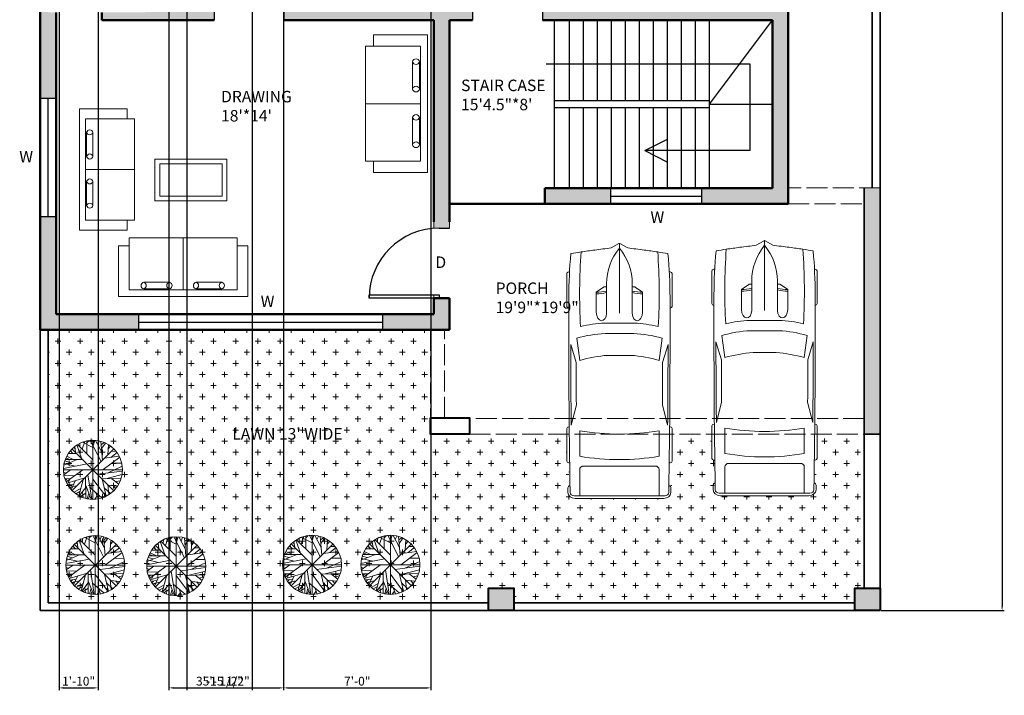
# Model space of a CAD drawing. Units: inches. Extents: x 2101 to 2663, y 1144 to 2069.
# Tile 1 of 4: x 2101 to 2663, y 1144 to 1530. Entities that reach past the tile are written whole.
import ezdxf

# ---------------------------------------------------------------- set-up
doc = ezdxf.new("R2010")
doc.units = ezdxf.units.IN
doc.linetypes.add('ACAD_ISO02W100', pattern=[15, 12, -3])
for name, color, linetype, lineweight in [('A-ANNO-DIMS', 2, 'Continuous', 18), ('A-ANNO-TEXT', 7, 'Continuous', 18), ('A-AREA-IDEN', 7, 'Continuous', 25), ('A-COLS', 7, 'Continuous', 40), ('A-FLOR-STRS', 7, 'Continuous', 25), ('A-WALL-OVHD', 240, 'ACAD_ISO02W100', 18), ('A-WALL-PATT', 240, 'Continuous', 13), ('C-PKNG-VEHI', 142, 'Continuous', 18), ('C-PROP', 7, 'Continuous', 35), ('door', 52, 'Continuous', 25), ('fur', 142, 'Continuous', 18), ('L-PLNT-PATT', 92, 'Continuous', 13), ('tree', 90, 'Continuous', 18), ('wall', 240, 'Continuous', 50), ('win', 150, 'Continuous', 25)]:
    doc.layers.add(name, color=color, linetype=linetype, lineweight=lineweight)
doc.styles.get("Standard").update_dxf_attribs({"font": 'arial.ttf'})
doc.dimstyles.new('ISO-25', dxfattribs={"dimtxt": 5, "dimasz": 2.5, "dimexe": 1.25, "dimexo": 0.625, "dimtad": 1, "dimdec": 0, "dimlunit": 4, "dimtxsty": 'Standard', "dimcen": 2.5, "dimadec": 0, "dimazin": 0, "dimtfac": 1, "dimtdec": 0, "dimtmove": 0, "dimatfit": 3, "dimfxl": 1, "dimarcsym": 0})

# ---------------------------------------------------------------- blocks, each defined once
blk = doc.blocks.new('*U6')
for p, q in [((0, 59.9996), (0, -60)), ((-43.8768, 36.4326), (-44.405, 40.2696)), ((42, 42), (-42, -42)), ((42, -42), (-42, 42)), ((-40.1797, 44.558), (-36.4825, 43.2038)), ((-37.0107, 47.0408), (-35.25, 35.5298)), ((-32.6092, 50.4264), (-23.2782, 23.5674)), ((-31.2008, 51.1035), (-0.2149, 20.1818)), ((-26.4472, 46.5894), (-26.2712, 53.8116)), ((-22.0458, 42.0753), (-16.5881, 57.6486)), ((-21.1656, 55.8436), (-0.0388, 45.0094)), ((-12.5388, 54.9406), (-7.9613, 59.4546)), ((-12.3627, 32.1443), (-12.5388, 58.7776)), ((-5.3205, 59.6806), (16.5105, 16.7963)), ((2.426, 54.9406), (-1.4472, 59.9056)), ((0.4894, 48.6208), (3.6584, 59.6806)), ((18.2711, 35.5298), (5.419, 59.6806)), ((9.8203, 51.5549), (12.8133, 58.5516)), ((19.6795, 19.5047), (16.3344, 57.6486)), ((17.0387, 51.1035), (23.2006, 55.1666)), ((17.7429, 43.6552), (25.4894, 54.2636)), ((31.6513, 50.8778), (30.2429, 30.5643)), ((31.1232, 42.5267), (35.8767, 48.1693)), ((-32.2571, 20.6333), (-59.1937, 9.348)), ((-56.0247, 20.859), (-20.8134, 20.859)), ((-54.7923, 24.4702), (-47.75, 21.0847)), ((-53.2078, 27.4044), (-40.1797, 20.859)), ((-49.8627, 32.8214), (-32.7853, 32.8214)), ((-45.8134, 38.2383), (-40.5318, 33.0471)), ((54.3626, 25.3731), (20.9119, 0.3198)), ((23.3767, 23.3417), (53.3063, 27.4044)), ((36.2288, 25.1474), (48.9049, 35.0784)), ((37.1091, 37.1098), (46.6161, 37.5612)), ((-59.7219, 2.8025), (-12.0106, 12.0565)), ((-58.6656, 12.7336), (-35.9543, 7.5424)), ((-57.081, 17.9248), (-47.0458, 14.7649)), ((-54.6162, -24.7335), (-20.2853, 0.0941)), ((29.3626, -6.6771), (59.4682, 7.091)), ((38.5175, 13.4107), (58.2359, 13.6364)), ((-60, 0), (60, 0)), ((-59.7219, -4.8714), (-54.2641, -6.6771)), ((-45.2853, -0.1316), (-59.0177, -10.0627)), ((-58.4895, -12.3197), (-36.4825, -11.6426)), ((-57.081, -18.4138), (-45.2853, -17.9624)), ((-52.6797, -18.188), (-55.4966, -22.0251)), ((-53.2078, -27.442), (-16.7641, -16.6081)), ((-47.2219, -19.3166), (-50.2148, -26.3135)), ((-14.8275, -15.0282), (-14.6515, -57.6865)), ((-10.074, -10.0627), (-2.5036, -59.7178)), ((-0.0388, -19.0909), (25.8415, -53.8495)), ((9.2922, -9.1598), (59.6443, -2.8401)), ((18.6232, -18.6394), (26.7218, -53.3981)), ((18.7992, -18.6394), (57.3556, -17.2853)), ((26.3697, -18.4138), (58.9401, -9.8369)), ((38.1654, -18.188), (52.426, -29.0219)), ((-38.9472, -29.0219), (-51.4472, -30.6018)), ((-46.5177, -30.1504), (-49.5106, -33.536)), ((-32.4331, -32.4075), (-48.1021, -35.5674)), ((-43.7008, -34.6645), (-46.6937, -37.373)), ((-35.9543, -22.4765), (-44.0529, -40.5329)), ((-24.6867, -37.8244), (-38.7712, -45.7241)), ((-19.9331, -20.2194), (-28.5599, -52.721)), ((-14.6515, -36.2445), (-27.6797, -52.9467)), ((-14.6515, -32.1818), (-3.912, -59.4922)), ((-6.2008, -36.2445), (17.919, -57.0094)), ((22.8485, -36.4702), (35.3485, -48.4326)), ((30.419, -30.1504), (32.3556, -50.0125)), ((31.4753, -31.279), (49.6091, -33.3103)), ((41.5105, -32.6332), (46.088, -38.0501)), ((45.9119, -24.0564), (55.595, -22.2508)), ((-26.2712, -43.9185), (-34.7219, -48.6583)), ((-14.6515, -47.3041), (-25.0388, -54.3009)), ((-21.5177, -45.4984), (-19.9331, -56.1065)), ((-8.4895, -47.5298), (-11.4825, -58.5893)), ((-6.3768, -52.721), (-9.3698, -58.815)), ((8.4119, -53.1724), (3.8344, -59.4922)), ((5.9471, -46.6269), (10.5246, -58.5893)), ((24.7852, -44.8213), (23.0246, -54.978))]:
    blk.add_line(p, q)
blk.add_circle((0, 0), 60)
blk = doc.blocks.new('*U2')
for p, q in [((0, 0), (0, -6)), ((40, 0), (40, -6))]:
    blk.add_line(p, q)
blk.add_lwpolyline([(0, 0), (0, 40), (1.75, 40), (1.75, 0)], close=True)
blk.add_arc((0, 0), 40, 0, 90)
blk = doc.blocks.new('*U8')
for p, q in [((21.1, 37.41), (21.1, 36.83)), ((46.55, 38.89), (22.35, 38.89)), ((47.8, 37.39), (47.8, 37.41)), ((135.45, 37.07), (135.45, 37.41)), ((136.7, 38.89), (160.9, 38.89)), ((162.15, 37.41), (162.15, 36.77)), ((70.03, 31.54), (86.41, 29.35)), ((87.99, 31.87), (74.76, 35.92)), ((134.31, 35.6), (119.29, 31.78)), ((138.42, 29.35), (157.25, 29.35)), ((186.47, 29.35), (167.01, 29.35)), ((186.47, -33.5), (186.47, 33.5)), ((188.4, -32.76), (188.4, 32.76)), ((164.52, 26.39), (164.52, -26.39)), ((32.27, 11.63), (36.13, 17.17)), ((36.13, 17.17), (50.94, 17.17)), ((29.77, 9.51), (51.68, 9.51)), ((32.12, 9.51), (32.12, 11.15)), ((58.92, -10.77), (58.92, 10.77)), ((66.55, -10.53), (66.55, 10.53)), ((82.74, 8.5), (82.74, -8.5)), ((186.47, -10.53), (186.47, 10.53)), ((3.27, 6.13), (0.1, 0.41)), ((0, 0), (51.68, 0)), ((0.1, -0.41), (3.27, -6.13)), ((29.77, -9.51), (51.68, -9.51)), ((32.12, -9.51), (32.12, -11.15)), ((32.27, -11.63), (36.13, -17.17)), ((36.13, -17.17), (50.94, -17.17)), ((86.41, -29.35), (70.03, -31.54)), ((87.99, -31.87), (74.76, -35.92)), ((134.31, -35.6), (119.29, -31.78)), ((157.25, -29.35), (138.42, -29.35)), ((167.01, -29.35), (186.47, -29.35)), ((21.1, -37.41), (21.1, -36.83)), ((46.55, -38.89), (22.35, -38.89)), ((47.8, -37.39), (47.8, -37.41)), ((135.45, -37.07), (135.45, -37.41)), ((136.7, -38.89), (160.9, -38.89)), ((162.15, -37.41), (162.15, -36.77))]:
    blk.add_line(p, q)
for centre, major_axis, ratio, start_param, end_param in [((41.19, -490.86), (0, 528.23), 0.842304, 0.00281, 0.075598), ((22.35, 37.41), (0, -1.48), 0.842304, 3.141593, 4.712389), ((64.48, -10555.62), (0, 10593.03), 0.842304, -0.013397, 0.002797), ((46.55, 37.41), (0, 1.48), 0.842304, -1.570796, 0), ((136.7, 37.41), (0, -1.48), 0.842304, 3.141593, 4.712389), ((160.9, 37.41), (0, 1.48), 0.842304, -1.570796, 0), ((180.63, 35.84), (0, 2.22), 0.842304, -0.013017, 1.249894), ((64.48, -10556.36), (0, 10595.31), 0.842304, -0.013397, -0.013017), ((183.98, 33.5), (0, -2.96), 0.842304, 1.570796, 3.128196), ((183.98, 32.76), (0, -5.25), 0.842304, 1.570796, 3.128196), ((266.03, -27.52), (0, 313.31), 0.842304, 1.367076, 1.39176), ((37.47, -593.96), (0, -623.33), 0.842304, 3.096046, 3.200911), ((135.29, 5.39), (0, 81.77), 0.842304, 1.245306, 1.50788), ((64.48, -10555.62), (0, -10591.55), 0.842304, 3.133765, 3.140441), ((149.6, 2.8), (0, -79.58), 0.842304, 4.372215, 4.640744), ((95.79, -3666.35), (0, -3698.24), 0.842304, 3.134049, 3.144098), ((17.08, 0), (0, 147.02), 0.842304, 4.511394, 4.913384), ((35.91, 0), (0, 147.02), 0.842304, 4.511394, 4.913384), ((167.01, 26.39), (0, 2.96), 0.842304, 0, 1.570796), ((259.18, -27.52), (0, -305.3), 0.842304, 4.528606, 4.561838), ((134.4, 5.39), (0, -89.78), 0.842304, 4.449482, 4.652344), ((-204.49, 52.4), (0, -250.96), 0.842304, 1.385369, 1.434372), ((13.04, 17.01), (0, 27.42), 0.842304, 4.435146, 4.718221), ((14.2, 17.01), (0, 27.42), 0.842304, 4.435146, 4.718221), ((50.79, 13.34), (6.34, -0.36), 0.603834, -1.395552, 1.581315), ((29.77, -46.66), (0, 56.17), 0.842304, 0, 0.590319), ((32.75, 11.15), (0, 0.74), 0.842304, 0.879714, 1.570796), ((0.62, 0), (0, -0.74), 0.842304, 4.131459, 5.293319), ((-204.49, -52.4), (0, 250.96), 0.842304, -1.434372, -1.385369), ((29.77, 46.66), (0, 56.17), 0.842304, 2.551274, 3.141593), ((32.75, -11.15), (0, -0.74), 0.842304, 4.712389, 5.403472), ((13.04, -17.01), (0, -27.42), 0.842304, 1.564964, 1.848039), ((14.2, -17.01), (0, -27.42), 0.842304, 1.564964, 1.848039), ((134.4, -5.39), (0, -89.78), 0.842304, -1.510751, -1.307889), ((135.29, -5.39), (0, -81.77), 0.842304, -1.50788, -1.245306), ((149.6, -2.8), (0, -79.58), 0.842304, -1.499151, -1.230623), ((259.18, 27.52), (0, 305.3), 0.842304, 1.721348, 1.754579), ((266.03, 27.52), (0, 313.31), 0.842304, 1.749832, 1.774517), ((37.47, 593.96), (0, -623.33), 0.842304, -0.059319, 0.045547), ((167.01, -26.39), (0, -2.96), 0.842304, 4.712389, 6.283185), ((41.19, 490.86), (0, -528.23), 0.842304, -0.075598, -0.00281), ((64.48, 10555.62), (0, -10591.55), 0.842304, 0.001152, 0.007828), ((95.79, 3666.35), (0, -3698.24), 0.842304, -0.002505, 0.007544), ((183.98, -33.5), (0, 2.96), 0.842304, 3.15499, 4.712389), ((183.98, -32.76), (0, -5.25), 0.842304, 0.013397, 1.570796), ((22.35, -37.41), (0, 1.48), 0.842304, 1.570796, 3.141593), ((64.48, 10555.62), (0, 10593.03), 0.842304, 3.138796, 3.15499), ((46.55, -37.41), (0, -1.48), 0.842304, 0, 1.570796), ((136.7, -37.41), (0, -1.48), 0.842304, -1.570796, 0), ((160.9, -37.41), (0, 1.48), 0.842304, 3.141593, 4.712389), ((180.63, -35.84), (0, -2.22), 0.842304, -1.249894, 0.013017), ((64.48, 10556.36), (0, 10595.31), 0.842304, 3.15461, 3.15499)]:
    blk.add_ellipse(centre, major_axis=major_axis, ratio=ratio, start_param=start_param, end_param=end_param)
at = {"extrusion": (0, 0, -1)}
blk.add_ellipse((50.79, -13.34), major_axis=(6.34, 0.36), ratio=0.603834, start_param=-1.395552, end_param=1.581315, dxfattribs=at)
blk = doc.blocks.new('*D10')
at = {"layer": 'A-ANNO-DIMS', "color": 0, "lineweight": -2, "transparency": 16777216}
for p, q in [((2593.02, 2003.65), (2663.42, 2003.65)), ((2662.17, 2001.15), (2662.17, 1194.65)), ((2593.02, 1192.15), (2663.42, 1192.15))]:
    blk.add_line(p, q, dxfattribs=at)
at = {"layer": 'A-ANNO-DIMS', "color": 0, "lineweight": 100, "transparency": 16777216}
for points in [[(2661.75, 2001.15), (2662.59, 2001.15), (2662.17, 2003.65)], [(2661.75, 1194.65), (2662.59, 1194.65), (2662.17, 1192.15)]]:
    blk.add_solid(points, dxfattribs=at)
at = {"layer": 'Defpoints', "color": 0, "lineweight": 100, "transparency": 16777216}
for p in [(2592.39, 2003.65), (2592.39, 1192.15), (2662.17, 1192.15)]:
    blk.add_point(p, dxfattribs=at)
at = {"layer": 'A-ANNO-DIMS', "color": 0, "transparency": 16777216, "insert": (2658.99, 1597.9), "char_height": 5, "attachment_point": 5, "rotation": 90}
blk.add_mtext('67\'-8"', dxfattribs=at)
blk = doc.blocks.new('*D31')
at = {"layer": 'A-ANNO-DIMS', "color": 0, "lineweight": -2, "transparency": 16777216}
for p, q in [((2196.07, 1776.74), (2196.07, 1146.75)), ((2233.58, 1776.74), (2233.58, 1146.75)), ((2198.57, 1148), (2231.08, 1148))]:
    blk.add_line(p, q, dxfattribs=at)
at = {"layer": 'A-ANNO-DIMS', "color": 0, "lineweight": 100, "transparency": 16777216}
for points in [[(2198.57, 1148.42), (2198.57, 1147.58), (2196.07, 1148)], [(2231.08, 1148.42), (2231.08, 1147.58), (2233.58, 1148)]]:
    blk.add_solid(points, dxfattribs=at)
at = {"layer": 'Defpoints', "color": 0, "lineweight": 100, "transparency": 16777216}
for p in [(2196.07, 1777.37), (2233.58, 1777.37), (2233.58, 1148)]:
    blk.add_point(p, dxfattribs=at)
at = {"layer": 'A-ANNO-DIMS', "color": 0, "transparency": 16777216, "insert": (2214.83, 1151.21), "char_height": 5, "attachment_point": 5}
blk.add_mtext('3\'-1 1/2"', dxfattribs=at)
blk = doc.blocks.new('*D32')
at = {"layer": 'A-ANNO-DIMS', "color": 0, "lineweight": -2, "transparency": 16777216}
for p, q in [((2123.19, 1725.57), (2123.19, 1146.75)), ((2145.39, 1725.57), (2145.39, 1146.75)), ((2125.69, 1148), (2142.89, 1148))]:
    blk.add_line(p, q, dxfattribs=at)
at = {"layer": 'A-ANNO-DIMS', "color": 0, "lineweight": 100, "transparency": 16777216}
for points in [[(2125.69, 1148.42), (2125.69, 1147.58), (2123.19, 1148)], [(2142.89, 1148.42), (2142.89, 1147.58), (2145.39, 1148)]]:
    blk.add_solid(points, dxfattribs=at)
at = {"layer": 'Defpoints', "color": 0, "lineweight": 100, "transparency": 16777216}
for p in [(2123.19, 1726.19), (2145.39, 1726.19), (2145.39, 1148)]:
    blk.add_point(p, dxfattribs=at)
at = {"layer": 'A-ANNO-DIMS', "color": 0, "transparency": 16777216, "insert": (2134.29, 1151.18), "char_height": 5, "attachment_point": 5}
blk.add_mtext('1\'-10"', dxfattribs=at)
blk = doc.blocks.new('*D34')
at = {"layer": 'A-ANNO-DIMS', "color": 0, "lineweight": -2, "transparency": 16777216}
for p, q in [((2185.89, 1947.53), (2185.89, 1146.75)), ((2251.48, 1947.53), (2251.48, 1146.75)), ((2188.39, 1148), (2248.98, 1148))]:
    blk.add_line(p, q, dxfattribs=at)
at = {"layer": 'A-ANNO-DIMS', "color": 0, "lineweight": 100, "transparency": 16777216}
for points in [[(2188.39, 1148.42), (2188.39, 1147.58), (2185.89, 1148)], [(2248.98, 1148.42), (2248.98, 1147.58), (2251.48, 1148)]]:
    blk.add_solid(points, dxfattribs=at)
at = {"layer": 'Defpoints', "color": 0, "lineweight": 100, "transparency": 16777216}
for p in [(2185.89, 1948.15), (2251.48, 1948.15), (2251.48, 1148)]:
    blk.add_point(p, dxfattribs=at)
at = {"layer": 'A-ANNO-DIMS', "color": 0, "transparency": 16777216, "insert": (2218.69, 1151.21), "char_height": 5, "attachment_point": 5}
blk.add_mtext('5\'-5 1/2"', dxfattribs=at)
blk = doc.blocks.new('*D35')
at = {"layer": 'A-ANNO-DIMS', "color": 0, "lineweight": -2, "transparency": 16777216}
for p, q in [((2251.48, 1947.53), (2251.48, 1146.75)), ((2335.68, 1947.53), (2335.68, 1146.75)), ((2253.98, 1148), (2333.18, 1148))]:
    blk.add_line(p, q, dxfattribs=at)
at = {"layer": 'A-ANNO-DIMS', "color": 0, "lineweight": 100, "transparency": 16777216}
for points in [[(2253.98, 1148.42), (2253.98, 1147.58), (2251.48, 1148)], [(2333.18, 1148.42), (2333.18, 1147.58), (2335.68, 1148)]]:
    blk.add_solid(points, dxfattribs=at)
at = {"layer": 'Defpoints', "color": 0, "lineweight": 100, "transparency": 16777216}
for p in [(2251.48, 1948.15), (2335.68, 1948.15), (2335.68, 1148)]:
    blk.add_point(p, dxfattribs=at)
at = {"layer": 'A-ANNO-DIMS', "color": 0, "transparency": 16777216, "insert": (2293.58, 1151.18), "char_height": 5, "attachment_point": 5}
blk.add_mtext('7\'-0"', dxfattribs=at)

msp = doc.modelspace()

# ---------------------------------------------------------------- hatches: boundary and pattern name
at = {"layer": 'A-WALL-PATT'}
h = msp.add_hatch(color=256, dxfattribs=at)
h.dxf.hatch_style = 1
h.paths.add_polyline_path([(2305.89, 1705.85), (2299.89, 1705.85), (2296.89, 1705.85), (2296.89, 1703.65), (2167.89, 1703.65), (2167.89, 1694.65), (2305.89, 1694.65)])
h.paths.add_polyline_path([(2305.89, 1804.15), (2121.39, 1804.15), (2121.39, 1799.65), (2296.89, 1799.65), (2296.89, 1775.65), (2296.89, 1745.74, -0.01877), (2299.89, 1745.85), (2305.89, 1745.85)])
h.paths.add_polyline_path([(2319.05, 1801.15, -0.01877), (2319.16, 1804.15), (2305.89, 1804.15), (2305.89, 1795.15), (2319.05, 1795.15)])
h.paths.add_polyline_path([(2365.89, 1804.15), (2359.05, 1804.15), (2359.05, 1801.15), (2359.05, 1795.15), (2365.89, 1795.15)])
h.paths.add_polyline_path([(2370.39, 1795.15), (2365.89, 1795.15), (2365.89, 1748.72), (2370.39, 1748.72)])
h.paths.add_polyline_path([(2305.89, 1694.65), (2296.89, 1694.65), (2296.89, 1656.63), (2305.89, 1656.63)])
h.paths.add_polyline_path([(2176.89, 1694.65), (2167.89, 1694.65), (2167.89, 1679.51), (2176.89, 1679.51)])
h.paths.add_polyline_path([(2134.3, 1610.65), (2116.89, 1610.65), (2116.89, 1606.15), (2134.3, 1606.15)])
h.paths.add_polyline_path([(2176.89, 1622.19), (2167.89, 1622.19), (2167.89, 1610.65), (2154.79, 1610.65), (2154.79, 1606.15), (2176.89, 1606.15)])
h.paths.add_polyline_path([(2176.89, 1606.15), (2172.39, 1606.15), (2172.39, 1534.15), (2147.63, 1534.15), (2147.63, 1529.65), (2176.89, 1529.65)])
h.paths.add_polyline_path([(2211.7, 1535.65), (2211.7, 1538.65), (2176.89, 1538.65), (2176.89, 1529.65), (2211.7, 1529.65)])
h.paths.add_polyline_path([(2116.89, 1606.15), (2112.39, 1606.15), (2112.39, 1529.65), (2121.39, 1529.65), (2121.39, 1534.15), (2116.89, 1534.15)])
h.paths.add_polyline_path([(2121.39, 1529.65), (2112.39, 1529.65), (2112.39, 1485), (2121.39, 1485)])
h.paths.add_polyline_path([(2359.39, 1535.65), (2359.39, 1538.65), (2314.89, 1538.65), (2251.59, 1538.65, -0.01877), (2251.7, 1535.65), (2251.7, 1529.65), (2359.39, 1529.65)])
h.paths.add_polyline_path([(2305.89, 1575.46), (2296.89, 1575.46), (2296.89, 1538.65), (2305.89, 1538.65)])
h.paths.add_polyline_path([(2539.89, 1584.63), (2530.89, 1584.63), (2530.89, 1538.65), (2399.28, 1538.65, -0.01877), (2399.39, 1535.65), (2399.39, 1529.65), (2539.89, 1529.65)])
h.paths.add_polyline_path([(2346.39, 1370.88), (2340.39, 1370.88), (2337.39, 1370.88), (2337.39, 1361.65), (2308.27, 1361.65), (2308.27, 1352.65), (2346.39, 1352.65)])
h.paths.add_polyline_path([(2168.45, 1361.65), (2121.39, 1361.65), (2121.39, 1417.42), (2112.39, 1417.42), (2112.39, 1352.65), (2168.45, 1352.65)])
h.paths.add_polyline_path([(2346.39, 1529.65), (2337.39, 1529.65), (2337.39, 1414.47), (2337.39, 1410.77, -0.01877), (2340.39, 1410.88), (2346.39, 1410.88), (2346.39, 1414.47)])
h.paths.add_polyline_path([(2592.39, 1433.97), (2583.39, 1433.97), (2583.39, 1292.97), (2592.39, 1292.97)])
h.paths.add_polyline_path([(2592.39, 1204.95), (2583.39, 1204.95), (2583.39, 1196.65), (2578.02, 1196.65), (2578.02, 1192.15), (2592.39, 1192.15)])
h.paths.add_polyline_path([(2583.39, 1204.95), (2578.02, 1204.95), (2578.02, 1196.65), (2583.39, 1196.65)], flags=17)
h.paths.add_polyline_path([(2382.99, 1204.95), (2368.62, 1204.95), (2368.62, 1196.65), (2382.99, 1196.65)])
h.paths.add_polyline_path([(2382.99, 1196.65), (2368.62, 1196.65), (2368.62, 1192.15), (2382.99, 1192.15)])
h.paths.add_polyline_path([(2490.54, 1433.65), (2490.54, 1424.65), (2539.89, 1424.65), (2539.89, 1433.97), (2539.89, 1529.65), (2530.89, 1529.65), (2530.89, 1433.65)])
h.paths.add_polyline_path([(2438.35, 1424.65), (2438.35, 1433.65), (2400.84, 1433.65), (2400.84, 1424.65)])
at = {"layer": 'L-PLNT-PATT'}
h = msp.add_hatch(dxfattribs=at)
h.set_pattern_fill('CROSS', color=256)
edge = h.paths.add_edge_path()
edge.add_line((2413.32, 1292.97), (2357.76, 1292.97))
edge.add_line((2357.76, 1292.97), (2335.45, 1292.97))
edge.add_line((2335.45, 1292.97), (2335.45, 1302.44))
edge.add_line((2335.45, 1302.44), (2335.45, 1352.65))
edge.add_line((2335.45, 1352.65), (2116.89, 1352.65))
edge.add_line((2116.89, 1352.65), (2116.89, 1196.65))
edge.add_line((2116.89, 1196.65), (2368.62, 1196.65))
edge.add_line((2368.62, 1196.65), (2368.62, 1204.95))
edge.add_line((2368.62, 1204.95), (2382.99, 1204.95))
edge.add_line((2382.99, 1204.95), (2382.99, 1196.65))
edge.add_line((2382.99, 1196.65), (2578.02, 1196.65))
edge.add_line((2578.02, 1196.65), (2578.02, 1204.95))
edge.add_line((2578.02, 1204.95), (2583.39, 1204.95))
edge.add_line((2583.39, 1204.95), (2583.39, 1292.97))
edge.add_line((2583.39, 1292.97), (2556.5, 1292.97))
edge.add_line((2556.5, 1292.97), (2556.5, 1278.81))
edge.add_ellipse((2555.35, 1279.16), major_axis=(-1.15, 0), ratio=0.842304, start_angle=90, end_angle=180, ccw=False)
edge.add_ellipse((-5642.84, 1353.78), major_axis=(8198.19, 0), ratio=0.8423039, start_angle=-0.618643, end_angle=-0.528271, ccw=False)
edge.add_ellipse((2554.13, 1263.9), major_axis=(-1.72, 0), ratio=0.842304, start_angle=179.3718, end_angle=248.4648, ccw=False)
edge.add_ellipse((-5643.41, 1353.78), major_axis=(-8199.96, 0), ratio=0.8423039, start_angle=179.353446, end_angle=179.371763, ccw=False)
edge.add_ellipse((2551.75, 1261.3), major_axis=(-4.06, 0), ratio=0.842304, start_angle=90, end_angle=179.3534, ccw=False)
edge.add_line((2551.75, 1257.88), (2500.58, 1257.88))
edge.add_ellipse((2501.05, 1261.3), major_axis=(4.06, 0), ratio=0.842304, start_angle=180.6466, end_angle=270, ccw=False)
edge.add_ellipse((10696.21, 1353.78), major_axis=(8199.96, 0), ratio=0.8423039, start_angle=180.628237, end_angle=180.646554, ccw=False)
edge.add_ellipse((2498.66, 1263.9), major_axis=(1.72, 0), ratio=0.842304, start_angle=111.5352, end_angle=180.6282, ccw=False)
edge.add_ellipse((10695.64, 1353.78), major_axis=(-8198.19, 0), ratio=0.8423039, start_angle=0.528271, end_angle=0.646554, ccw=False)
edge.add_line((2497.94, 1278.2), (2497.03, 1278.2))
edge.add_ellipse((2497.45, 1279.16), major_axis=(1.15, 0), ratio=0.842304, start_angle=180, end_angle=270, ccw=False)
edge.add_line((2496.3, 1279.16), (2496.3, 1292.97))
edge.add_line((2496.3, 1292.97), (2473.52, 1292.97))
edge.add_line((2473.52, 1292.97), (2473.52, 1277.27))
edge.add_ellipse((2472.37, 1277.62), major_axis=(-1.15, 0), ratio=0.842304, start_angle=90, end_angle=180, ccw=False)
edge.add_ellipse((-5725.82, 1352.24), major_axis=(8198.19, 0), ratio=0.8423039, start_angle=-0.618643, end_angle=-0.528271, ccw=False)
edge.add_ellipse((2471.16, 1262.35), major_axis=(-1.72, 0), ratio=0.842304, start_angle=179.3718, end_angle=248.4648, ccw=False)
edge.add_ellipse((-5726.39, 1352.24), major_axis=(-8199.96, 0), ratio=0.8423039, start_angle=179.353446, end_angle=179.371763, ccw=False)
edge.add_ellipse((2468.77, 1259.76), major_axis=(-4.06, 0), ratio=0.842304, start_angle=90, end_angle=179.3534, ccw=False)
edge.add_line((2468.77, 1256.34), (2417.6, 1256.34))
edge.add_ellipse((2418.07, 1259.76), major_axis=(4.06, 0), ratio=0.842304, start_angle=180.6466, end_angle=270, ccw=False)
edge.add_ellipse((10613.23, 1352.24), major_axis=(-8199.96, 0), ratio=0.8423039, start_angle=0.628237, end_angle=0.646554, ccw=False)
edge.add_ellipse((2415.68, 1262.35), major_axis=(1.72, 0), ratio=0.842304, start_angle=111.5352, end_angle=180.6282, ccw=False)
edge.add_ellipse((10612.66, 1352.24), major_axis=(-8198.19, 0), ratio=0.8423039, start_angle=0.528271, end_angle=0.646554, ccw=False)
edge.add_line((2414.96, 1276.65), (2414.05, 1276.65))
edge.add_ellipse((2414.47, 1277.62), major_axis=(1.15, 0), ratio=0.842304, start_angle=180, end_angle=270, ccw=False)
edge.add_line((2413.32, 1277.62), (2413.32, 1292.97))

# ---------------------------------------------------------------- linework, layer by layer
at = {"layer": 'A-COLS'}
for points in [[(2335.45, 1302.44), (2357.76, 1302.44), (2357.76, 1292.97), (2335.45, 1292.97)], [(2382.99, 1192.15), (2368.62, 1192.15), (2368.62, 1204.95), (2382.99, 1204.95)], [(2592.39, 1192.15), (2578.02, 1192.15), (2578.02, 1204.95), (2592.39, 1204.95)]]:
    msp.add_lwpolyline(points, close=True, dxfattribs=at)
at = {"layer": 'A-FLOR-STRS'}
for p, q in [((2406.39, 1433.65), (2406.39, 1529.65)), ((2414.89, 1483.65), (2414.89, 1529.65)), ((2422.89, 1483.65), (2422.89, 1529.65)), ((2430.89, 1483.65), (2430.89, 1529.65)), ((2438.89, 1483.65), (2438.89, 1529.65)), ((2446.89, 1483.65), (2446.89, 1529.65)), ((2454.89, 1483.65), (2454.89, 1529.65)), ((2462.89, 1483.65), (2462.89, 1529.65)), ((2470.89, 1483.65), (2470.89, 1529.65)), ((2478.89, 1483.65), (2478.89, 1529.65)), ((2486.89, 1483.65), (2486.89, 1529.65)), ((2494.89, 1433.65), (2494.89, 1529.65)), ((2494.89, 1481.65), (2530.89, 1529.65)), ((2401.63, 1504.75), (2517.89, 1504.75)), ((2517.89, 1504.75), (2517.89, 1455.17)), ((2494.89, 1483.65), (2406.39, 1483.65)), ((2494.89, 1481.65), (2530.89, 1481.65)), ((2494.89, 1479.65), (2406.39, 1479.65)), ((2414.89, 1433.65), (2414.89, 1479.65)), ((2422.89, 1433.65), (2422.89, 1479.65)), ((2430.89, 1433.65), (2430.89, 1479.65)), ((2438.89, 1433.65), (2438.89, 1479.65)), ((2446.89, 1433.65), (2446.89, 1479.65)), ((2454.89, 1433.65), (2454.89, 1479.65)), ((2462.89, 1433.65), (2462.89, 1479.65)), ((2470.89, 1433.65), (2470.89, 1479.65)), ((2478.89, 1433.65), (2478.89, 1479.65)), ((2486.89, 1433.65), (2486.89, 1479.65)), ((2457.97, 1455.17), (2470.89, 1461.73)), ((2517.89, 1455.17), (2457.97, 1455.17)), ((2457.97, 1455.17), (2470.89, 1448.61)), ((2530.89, 1433.65), (2494.89, 1433.65))]:
    msp.add_line(p, q, dxfattribs=at)
at = {"layer": 'A-WALL-OVHD'}
msp.add_line((2587.89, 1448.02), (2587.89, 1433.97), dxfattribs=at)
for points in [[(2592.39, 1424.65), (2592.39, 1433.97), (2539.89, 1433.97), (2539.89, 1424.65), (2583.39, 1424.65)], [(2337.39, 1414.47), (2337.39, 1410.77)], [(2346.39, 1410.88), (2346.39, 1414.47)], [(2337.39, 1372.63), (2337.39, 1370.88), (2346.39, 1370.88)]]:
    msp.add_lwpolyline(points, dxfattribs=at)
for points in [[(2335.45, 1302.44), (2343.37, 1302.44), (2343.37, 1352.65), (2335.45, 1352.65)], [(2357.76, 1292.97), (2583.39, 1292.97), (2583.39, 1302.03), (2357.76, 1302.03)]]:
    msp.add_lwpolyline(points, close=True, dxfattribs=at)
at = {"layer": 'C-PROP'}
for p, q in [((2592.39, 1433.97), (2592.39, 2003.65)), ((2587.89, 1999.15), (2587.89, 1433.97)), ((2587.89, 1893.68), (2587.89, 1448.02)), ((2592.39, 1893.68), (2592.39, 1448.02)), ((2592.39, 1448.02), (2592.39, 1192.15)), ((2583.39, 1433.97), (2583.39, 1204.95)), ((2112.39, 1352.65), (2112.39, 1192.15)), ((2112.39, 1352.65), (2112.39, 1192.15)), ((2116.89, 1352.65), (2116.89, 1196.65)), ((2116.89, 1352.65), (2116.89, 1196.65)), ((2116.89, 1196.65), (2116.89, 1352.65)), ((2583.39, 1292.97), (2592.39, 1292.97)), ((2583.39, 1292.97), (2583.39, 1204.95)), ((2592.39, 1192.15), (2592.39, 1292.97)), ((2116.89, 1196.65), (2368.62, 1196.65)), ((2116.89, 1196.65), (2368.62, 1196.65)), ((2368.62, 1196.65), (2116.89, 1196.65)), ((2578.02, 1196.65), (2382.99, 1196.65)), ((2382.99, 1196.65), (2578.02, 1196.65)), ((2382.99, 1196.65), (2578.02, 1196.65)), ((2112.39, 1192.15), (2592.39, 1192.15)), ((2112.39, 1192.15), (2592.39, 1192.15))]:
    msp.add_line(p, q, dxfattribs=at)
at = {"layer": 'door'}
msp.add_line((2346.39, 1424.65), (2400.84, 1424.65), dxfattribs=at)
at = {"layer": 'fur'}
for p, q in [((2333.81, 1521.29), (2302.88, 1521.29)), ((2302.88, 1521.29), (2302.88, 1514.88)), ((2333.81, 1442.63), (2333.81, 1521.29)), ((2298.21, 1481.98), (2329.8, 1481.98)), ((2134.79, 1409.7), (2134.79, 1479.08)), ((2134.79, 1479.08), (2162.07, 1479.08)), ((2162.07, 1479.08), (2162.07, 1473.42)), ((2302.88, 1449.07), (2302.88, 1442.63)), ((2166.19, 1444.41), (2138.33, 1444.41)), ((2302.88, 1442.63), (2333.81, 1442.63)), ((2162.07, 1415.39), (2162.07, 1409.7)), ((2162.07, 1409.7), (2134.79, 1409.7)), ((2194.1, 1405.21), (2194.1, 1375.54)), ((2157.19, 1371.78), (2157.19, 1400.82)), ((2157.19, 1400.82), (2163.21, 1400.82)), ((2224.99, 1400.82), (2231.04, 1400.82)), ((2231.04, 1400.82), (2231.04, 1371.78)), ((2231.04, 1371.78), (2157.19, 1371.78))]:
    msp.add_line(p, q, dxfattribs=at)
for points in [[(2329.8, 1449.07), (2298.21, 1449.07), (2298.21, 1514.88), (2329.8, 1514.88)], [(2138.33, 1415.39), (2166.19, 1415.39), (2166.19, 1473.42), (2138.33, 1473.42)], [(2177.93, 1450.28), (2219.04, 1450.28), (2219.04, 1426.44), (2177.93, 1426.44)], [(2180.69, 1447.52), (2216.3, 1447.52), (2216.3, 1429.14), (2180.69, 1429.14)], [(2224.99, 1375.54), (2224.99, 1405.21), (2163.21, 1405.21), (2163.21, 1375.54)]]:
    msp.add_lwpolyline(points, close=True, dxfattribs=at)
for points in [[(2325.16, 1505.94), (2325.16, 1490.36)], [(2329.15, 1490.36), (2329.15, 1505.94)], [(2325.16, 1474.07), (2325.16, 1458.49)], [(2329.15, 1458.49), (2329.15, 1474.07)], [(2138.9, 1451.8), (2138.9, 1465.54)], [(2142.42, 1465.54), (2142.42, 1451.8)], [(2138.9, 1423.69), (2138.9, 1437.43)], [(2142.42, 1437.43), (2142.42, 1423.69)], [(2171.6, 1379.9), (2186.23, 1379.9)], [(2201.52, 1379.9), (2216.15, 1379.9)], [(2186.23, 1376.16), (2171.6, 1376.16)], [(2216.15, 1376.16), (2201.52, 1376.16)]]:
    msp.add_lwpolyline(points, dxfattribs=at)
for centre, radius, start, end in [((2327.16, 1505.63), 2.02, 8.6987, 171.3013), ((2327.16, 1506.52), 2.08, 196.4476, 343.5524), ((2327.16, 1489.94), 2.04, 11.8934, 168.1066), ((2327.16, 1490.78), 2.04, 191.9211, 348.0789), ((2327.16, 1473.76), 2.02, 8.6987, 171.3013), ((2327.16, 1474.66), 2.08, 196.4476, 343.5524), ((2140.66, 1465.27), 1.78, 8.6987, 171.3013), ((2140.66, 1466.06), 1.83, 196.4476, 343.5524), ((2327.16, 1458.07), 2.04, 11.8934, 168.1066), ((2327.16, 1458.91), 2.04, 191.9211, 348.0789), ((2140.66, 1451.43), 1.8, 11.8934, 168.1066), ((2140.66, 1452.17), 1.8, 191.9211, 348.0789), ((2140.66, 1437.16), 1.78, 8.6987, 171.3013), ((2140.66, 1437.95), 1.83, 196.4476, 343.5524), ((2140.66, 1423.32), 1.8, 11.8934, 168.1066), ((2140.66, 1424.07), 1.8, 191.9211, 348.0789), ((2171.89, 1378.03), 1.89, 98.6987, 261.3013), ((2171.05, 1378.03), 1.95, 286.4476, 73.5524), ((2186.62, 1378.03), 1.91, 101.8934, 258.1066), ((2185.83, 1378.03), 1.91, 281.9211, 78.0789), ((2201.81, 1378.03), 1.89, 98.6987, 261.3013), ((2200.97, 1378.03), 1.95, 286.4476, 73.5524), ((2216.54, 1378.03), 1.91, 101.8934, 258.1066), ((2215.75, 1378.03), 1.91, 281.9211, 78.0789)]:
    msp.add_arc(centre, radius, start, end, dxfattribs=at)
at = {"layer": 'wall'}
for p, q in [((2539.89, 1694.65), (2539.89, 1529.65)), ((2112.39, 1606.15), (2112.39, 1529.65)), ((2121.39, 1529.65), (2121.39, 1534.15)), ((2147.63, 1534.15), (2147.63, 1529.65)), ((2112.39, 1529.65), (2112.39, 1352.65)), ((2121.39, 1529.65), (2121.39, 1361.65)), ((2147.63, 1529.65), (2211.7, 1529.65)), ((2147.63, 1529.65), (2176.89, 1529.65)), ((2211.7, 1529.65), (2176.89, 1529.65)), ((2305.89, 1529.65), (2251.7, 1529.65)), ((2251.7, 1529.65), (2337.39, 1529.65)), ((2337.39, 1529.65), (2337.39, 1414.47)), ((2346.39, 1529.65), (2346.39, 1414.47)), ((2346.39, 1529.65), (2359.39, 1529.65)), ((2399.39, 1529.65), (2530.89, 1529.65)), ((2530.89, 1529.65), (2530.89, 1433.65)), ((2539.89, 1529.65), (2539.89, 1424.65)), ((2406.39, 1433.65), (2400.84, 1433.65)), ((2400.84, 1433.65), (2400.84, 1424.65)), ((2530.89, 1433.65), (2406.39, 1433.65)), ((2539.89, 1424.65), (2346.39, 1424.65)), ((2337.39, 1370.88), (2346.39, 1370.88)), ((2337.39, 1370.88), (2337.39, 1361.65)), ((2346.39, 1370.88), (2346.39, 1352.65)), ((2337.39, 1361.65), (2121.39, 1361.65)), ((2346.39, 1352.65), (2112.39, 1352.65))]:
    msp.add_line(p, q, dxfattribs=at)
at = {"layer": 'win'}
for p, q in [((2116.89, 1417.42), (2116.89, 1485)), ((2438.35, 1429.15), (2490.54, 1429.15)), ((2168.45, 1357.15), (2308.27, 1357.15))]:
    msp.add_line(p, q, dxfattribs=at)
for points in [[(2112.39, 1417.42), (2121.39, 1417.42), (2121.39, 1485), (2112.39, 1485)], [(2438.35, 1424.65), (2490.54, 1424.65), (2490.54, 1433.65), (2438.35, 1433.65)], [(2168.45, 1352.65), (2308.27, 1352.65), (2308.27, 1361.65), (2168.45, 1361.65)]]:
    msp.add_lwpolyline(points, close=True, dxfattribs=at)

# ---------------------------------------------------------------- block references
at = {"layer": 'C-PKNG-VEHI', "xscale": 0.7739235724712064, "yscale": 0.7739235724712064, "zscale": 0.7739235724712064, "rotation": 270}
for p in [(2443.42, 1402.14), (2526.4, 1403.69)]:
    msp.add_blockref('*U8', p, dxfattribs=at)
at = {"layer": 'door'}
for p in [(2211.7, 1535.65), (2359.39, 1535.65)]:
    msp.add_blockref('*U2', p, dxfattribs=at)
at = {"layer": 'door', "rotation": 90}
msp.add_blockref('*U2', (2340.39, 1370.88), dxfattribs=at)
at = {"layer": 'tree', "xscale": 0.2816711197250754, "yscale": 0.2816711197250754, "zscale": 0.2816711197250754}
for p in [(2142.5, 1272.69), (2143.86, 1218.24), (2190.14, 1217.55), (2267.73, 1218.33), (2312.52, 1218.33)]:
    msp.add_blockref('*U6', p, dxfattribs=at)

# ---------------------------------------------------------------- texts
at = {"layer": 'A-ANNO-TEXT', "char_height": 6.57, "attachment_point": 1}
for s, insert in [('W', (2100.4, 1454.97)), ('W', (2461.17, 1420.39)), ('D', (2338.24, 1394.63)), ('W', (2238.36, 1372.28))]:
    msp.add_mtext_dynamic_manual_height_columns(s, width=76.8305, gutter_width=32.84, heights=[0], dxfattribs=dict(at, insert=insert))
at = {"layer": 'A-AREA-IDEN', "attachment_point": 1}
for s, insert, char_height in [('STAIR CASE\\P15\'4.5"*8\'', (2352.93, 1495.74), 6.568), ("DRAWING\\P18'*14'", (2215.73, 1489.33), 6.568), ('PORCH\\P19\'9"*19\'9"', (2372.66, 1379.78), 6.5684), ("LAWN 13' WIDE", (2222.15, 1296.54), 6.5684)]:
    msp.add_mtext_dynamic_manual_height_columns(s, width=76.8305, gutter_width=32.84, heights=[0], dxfattribs=dict(at, insert=insert, char_height=char_height))

# ---------------------------------------------------------------- dimensions: what is measured, and where the dimension line sits
at = {"layer": 'A-ANNO-DIMS'}
dim = msp.add_linear_dim(base=(2662.16897098, 1192.1502194), p1=(2592.39296591, 2003.6502194), p2=(2592.39296591, 1192.1502194), angle=90, dimstyle='ISO-25', override={"dimclrd": 0, "dimclre": 0, "dimclrt": 0}, dxfattribs=at)
dim.commit()
dim.dimension.update_dxf_attribs({"geometry": '*D10', "text_midpoint": (2658.99110604, 1597.9002194)})
for base, p1, p2, picture, middle in [((2251.48, 1148), (2185.89, 1948.15), (2251.48, 1948.15), '*D34', (2218.69, 1151.21)), ((2335.68, 1148), (2251.48, 1948.15), (2335.68, 1948.15), '*D35', (2293.58, 1151.18)), ((2233.58, 1148), (2196.07, 1777.37), (2233.58, 1777.37), '*D31', (2214.83, 1151.21)), ((2145.39, 1148), (2123.19, 1726.19), (2145.39, 1726.19), '*D32', (2134.29, 1151.18))]:
    dim = msp.add_linear_dim(base=base, p1=p1, p2=p2, dimstyle='ISO-25', override={"dimdec": 1, "dimlfac": 1, "dimrnd": 0, "dimzin": 1, "dimdsep": 46, "dimlunit": 4, "dimfrac": 2}, dxfattribs=at)
    dim.commit()
    dim.dimension.update_dxf_attribs({"geometry": picture, "text_midpoint": middle})

doc.saveas('drawing.dxf')
